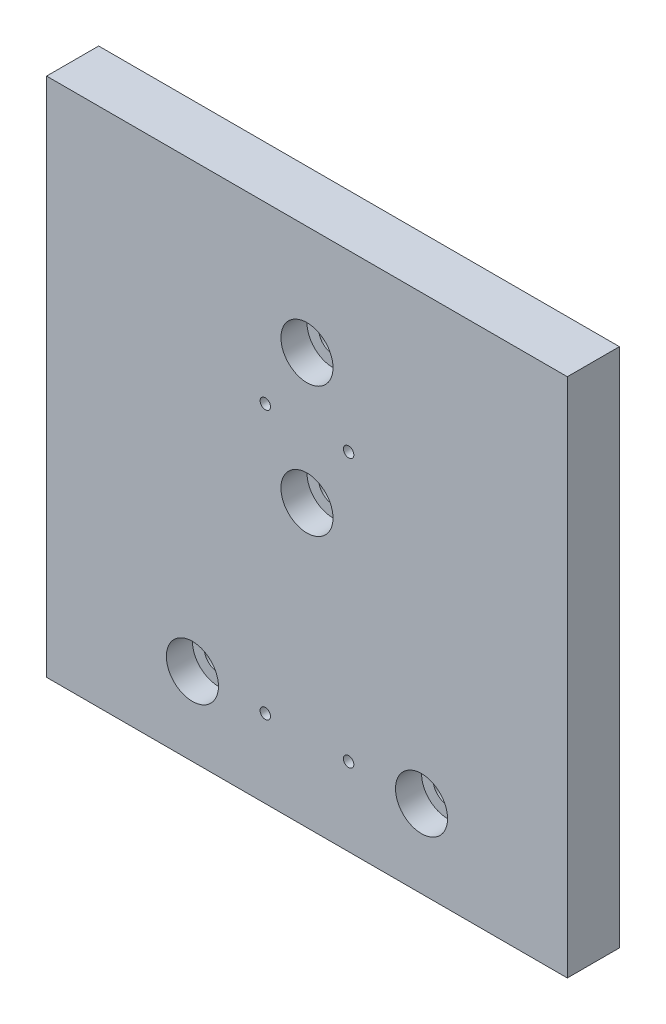
from build123d import *

# Parameters (mm, degrees)
BASE_PLATE_100X100X10_DEPTH  = 10
COUNTERBORE_SKETCH_R         = 5
COUNTERBORES_4X_10X5_DEPTH   = 5
CLEARANCE_HOLE_SKETCH_R      = 2.75
CLEARANCE_HOLES_4X_5_5_DEPTH = 12
SMALL_HOLE_SKETCH_R          = 1
SMALL_HOLES_4X_2X8_DEPTH     = 8
RECESS_SKETCH_R              = 2.5
RECESSES_2X_5X5_DEPTH        = 5
STEPPED_HOLE_SKETCH_R        = 1.5
STEPPED_HOLES_2X_3_DEPTH     = 70


with BuildPart() as part:
    # Base Plate Sketch → Base Plate 100x100x10 (new body)
    with BuildSketch(Plane.XY):
        Polygon((0, 0), (50, 0), (50, 100), (-50, 100), (-50, 0), align=None)
    extrude(amount=BASE_PLATE_100X100X10_DEPTH)

    # Counterbore Sketch → Counterbores 4x_10x5 (cut)
    with BuildSketch(Plane.XY.offset(10)):
        with Locations((0, 54)):
            Circle(COUNTERBORE_SKETCH_R)
        with Locations((0, 79)):
            Circle(COUNTERBORE_SKETCH_R)
        with Locations((22, 15)):
            Circle(COUNTERBORE_SKETCH_R)
        with Locations((-22, 15)):
            Circle(COUNTERBORE_SKETCH_R)
    extrude(amount=-COUNTERBORES_4X_10X5_DEPTH, mode=Mode.SUBTRACT)

    # Clearance Hole Sketch → Clearance Holes 4x_5.5 (cut)
    with BuildSketch(Plane.XY.offset(5)):
        with Locations((0, 79)):
            Circle(CLEARANCE_HOLE_SKETCH_R)
        with Locations((0, 54)):
            Circle(CLEARANCE_HOLE_SKETCH_R)
        with Locations((22, 15)):
            Circle(CLEARANCE_HOLE_SKETCH_R)
        with Locations((-22, 15)):
            Circle(CLEARANCE_HOLE_SKETCH_R)
    extrude(amount=-CLEARANCE_HOLES_4X_5_5_DEPTH, mode=Mode.SUBTRACT)

    # Small Hole Sketch → Small Holes 4x_2x8 (cut)
    with BuildSketch(Plane.XY.offset(10)):
        with Locations((8, 15)):
            Circle(SMALL_HOLE_SKETCH_R)
        with Locations((-8, 15)):
            Circle(SMALL_HOLE_SKETCH_R)
        with Locations((8, 66.5)):
            Circle(SMALL_HOLE_SKETCH_R)
        with Locations((-8, 66.5)):
            Circle(SMALL_HOLE_SKETCH_R)
    extrude(amount=-SMALL_HOLES_4X_2X8_DEPTH, mode=Mode.SUBTRACT)

    # Recess Sketch → Recesses 2x_5x5 (cut)
    with BuildSketch(Plane.XZ):
        with Locations(Location((-8, 5, 0), (0, 0, 270))):
            Circle(RECESS_SKETCH_R)
        with Locations(Location((8, 5, 0), (0, 0, 270))):
            Circle(RECESS_SKETCH_R)
    extrude(amount=-RECESSES_2X_5X5_DEPTH, mode=Mode.SUBTRACT)

    # Stepped Hole Sketch → Stepped Holes 2x_3 (cut)
    with BuildSketch(Plane.XZ):
        with Locations(Location((8, 5, 0), (0, 0, 270))):
            Circle(STEPPED_HOLE_SKETCH_R)
        with Locations(Location((-8, 5, 0), (0, 0, 270))):
            Circle(STEPPED_HOLE_SKETCH_R)
    extrude(amount=-STEPPED_HOLES_2X_3_DEPTH, mode=Mode.SUBTRACT)


solid = part.part
